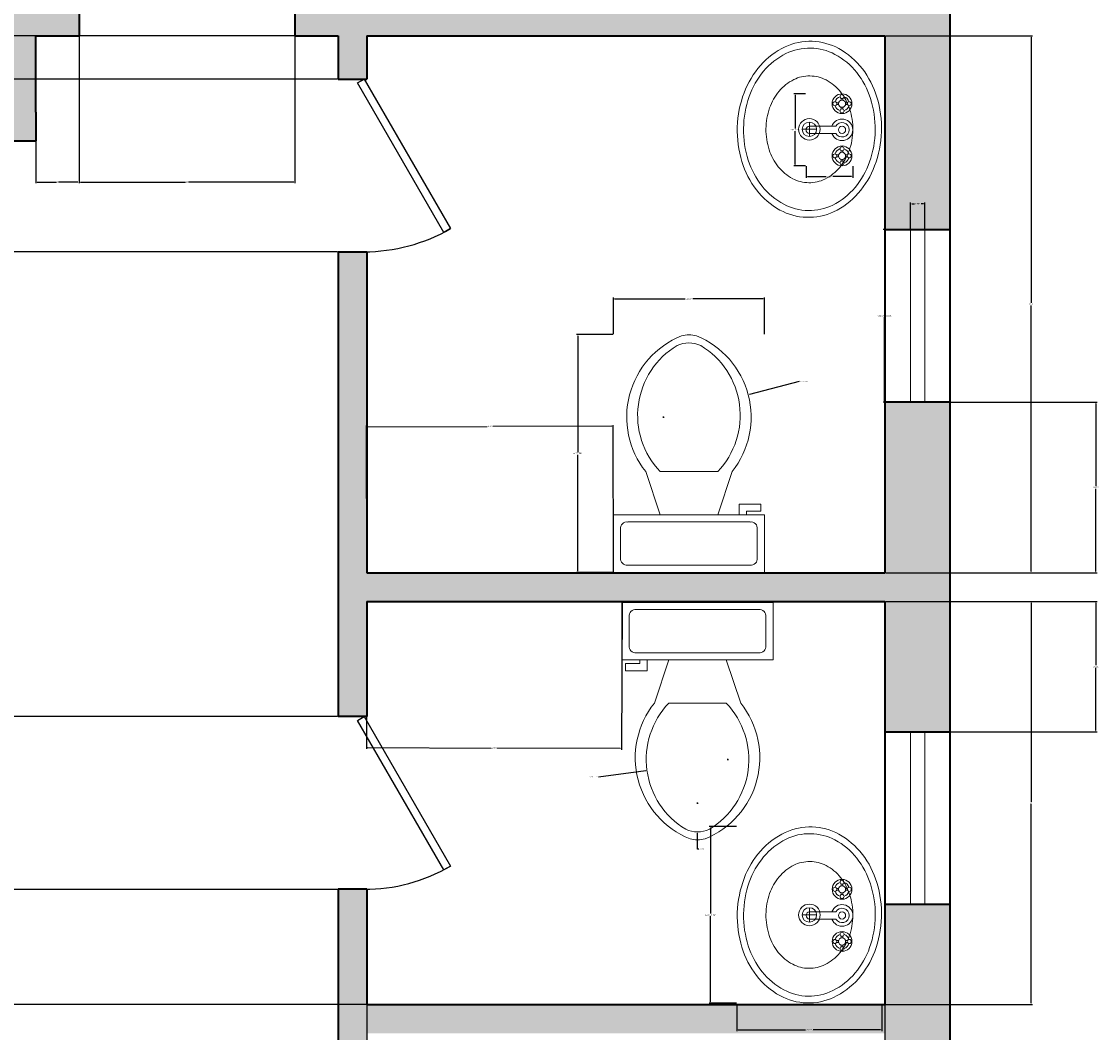
# Model space of a CAD drawing. Units: inches. Extents: x 1984 to 2284, y 2002 to 2421.
# Tile 3 of 4: x 2134 to 2284, y 2144 to 2285. Entities that reach past the tile are written whole.
import ezdxf

# ---------------------------------------------------------------- set-up
doc = ezdxf.new("R2010")
doc.units = ezdxf.units.IN
for name, color, linetype, lineweight in [('A-ANNO-DIMS', 2, 'Continuous', 18), ('A-DOOR', 3, 'Continuous', 25), ('A-FLOR-FIXT', 8, 'Continuous', 18), ('A-GLAZ', 4, 'Continuous', 18), ('A-WALL', 7, 'Continuous', 35)]:
    doc.layers.add(name, color=color, linetype=linetype, lineweight=lineweight)
doc.layers.add('A-WALL-PATT', color=18, linetype='Continuous', lineweight=13, true_color=0x000000)
doc.styles.get("Standard").update_dxf_attribs({"font": 'arial.ttf'})
doc.dimstyles.get("Standard").update_dxf_attribs({"dimtxt": 0.18, "dimasz": 0.18, "dimexe": 0.18, "dimexo": 0.0625, "dimgap": 0.09, "dimtad": 0, "dimtih": 1, "dimtoh": 1, "dimdec": 4, "dimzin": 0, "dimdsep": 46, "dimtxsty": 'Standard', "dimcen": 0.09, "dimadec": 0, "dimazin": 0, "dimtfac": 1, "dimtdec": 4, "dimtofl": 0, "dimtmove": 0, "dimatfit": 3, "dimfxl": 1, "dimtolj": 1, "dimtzin": 0, "dimarcsym": 0})

# ---------------------------------------------------------------- blocks, each defined once
blk = doc.blocks.new('Toilet - top')
for p, q in [((9.5, -6), (9.5, -2)), ((-10, -8.5), (-8, -8.5)), ((-10, -9.5), (-10, -8.5)), ((-8, -8.5), (-8, -8)), ((-7, -8), (-7, -9.5)), ((-4, -8), (-6, -14)), ((4, -8), (6, -14)), ((-7, -9.5), (-10, -9.5)), ((4, -14), (-4, -14))]:
    blk.add_line(p, q)
blk.add_lwpolyline([(10.5, -8), (10.5, 0), (-10.5, 0), (-10.5, -8)], close=True)
for points in [[(8.5, -1), (-8.5, -1)], [(-9.5, -2), (-9.5, -6)], [(-8.5, -7), (8.5, -7)]]:
    blk.add_lwpolyline(points)
for centre, radius, start, end in [((-8.62, -1.88), 0.884, 81.8699, 188.1301), ((8.62, -1.88), 0.884, 351.8699, 98.1301), ((-8.62, -6.12), 0.884, 171.8699, 278.1301), ((8.62, -6.12), 0.884, 261.8699, 8.1301), ((3.52, -21.58), 12.17, 141.4691, 247.9714), ((4.2, -21.82), 11.33, 136.3677, 238.9468), ((-3.52, -21.58), 12.17, 292.0284, 38.5307), ((-4.2, -21.82), 11.33, 301.053, 43.6321), ((0, -27.88), 4, 245.7318, 294.2682), ((0, -29), 4, 254.8605, 285.1395)]:
    blk.add_arc(centre, radius, start, end)
blk = doc.blocks.new('Sink - Oval top')
for p, q in [((-1, 0), (1, 0)), ((0, 1), (0, -1))]:
    blk.add_line(p, q)
for points in [[(-12.23, 0.39, 0.117634), (-11.46, -3.36, 0.104469), (-8.88, -6.8, 0.090016), (-5.08, -9.07, 0.08192), (-0.32, -10.02, 0.08192), (4.49, -9.38, 0.090016), (8.42, -7.36, 0.104469), (11.22, -4.09, 0.117634), (12.23, -0.39, 0.117634), (11.46, 3.36, 0.104469), (8.88, 6.8, 0.090016), (5.08, 9.07, 0.08192), (0.32, 10.02, 0.08192), (-4.49, 9.38, 0.090016), (-8.42, 7.36, 0.104469), (-11.22, 4.09, 0.117634)], [(-11.29, 0.16, 0.118622), (-10.52, -3.25, 0.104678), (-8.07, -6.36, 0.089562), (-4.54, -8.37, 0.081185), (-0.13, -9.15, 0.081185), (4.3, -8.49, 0.089562), (7.89, -6.58, 0.104678), (10.42, -3.55, 0.118622), (11.29, -0.16, 0.118622), (10.52, 3.25, 0.104678), (8.07, 6.36, 0.089562), (4.54, 8.37, 0.081185), (0.13, 9.15, 0.081185), (-4.3, 8.49, 0.089562), (-7.89, 6.58, 0.104678), (-10.42, 3.55, 0.118622)], [(-7.42, 0.08, 0.118283), (-6.91, -2.17, 0.104607), (-5.29, -4.21, 0.089718), (-2.97, -5.53, 0.081436), (-0.07, -6.04, 0.081436), (2.84, -5.59, 0.089718), (5.2, -4.33, 0.104607), (6.86, -2.32, 0.118283), (7.42, -0.08, 0.118283), (6.91, 2.17, 0.104607), (5.29, 4.21, 0.089718), (2.97, 5.53, 0.081436), (0.07, 6.04, 0.081436), (-2.84, 5.59, 0.089718), (-5.2, 4.33, 0.104607), (-6.86, 2.32, 0.118283)]]:
    blk.add_lwpolyline(points, format="xyb", close=True)
for radius in [1.5, 1]:
    blk.add_circle((0, 0), radius)
blk = doc.blocks.new('Faucet - Bathroom top')
for p, q in [((-4.107, 0.125), (-4.375, 0.125)), ((-3.75, 0.4788), (-3.75, 0.75)), ((-3.5, 0.482), (-3.5, 0.75)), ((-3.1461, 0.125), (-2.875, 0.125)), ((3.143, 0.125), (2.875, 0.125)), ((3.5, 0.4788), (3.5, 0.75)), ((3.75, 0.482), (3.75, 0.75)), ((4.1039, 0.125), (4.375, 0.125)), ((-4.1039, -0.125), (-4.375, -0.125)), ((-3.75, -0.4821), (-3.75, -0.75)), ((-3.5, -0.4789), (-3.5, -0.75)), ((-3.143, -0.125), (-2.875, -0.125)), ((-0.5, -0.8639), (-0.5, -4.5)), ((0.5, -4.5), (0.5, -0.8631)), ((3.1461, -0.125), (2.875, -0.125)), ((3.5, -0.4821), (3.5, -0.75)), ((3.75, -0.4789), (3.75, -0.75)), ((4.107, -0.125), (4.375, -0.125))]:
    blk.add_line(p, q)
for centre, radius in [((-3.625, 0), 1.375), ((-4.625, 0), 0.2795), ((-3.625, 0), 0.5), ((-3.625, 1), 0.2795), ((-2.625, 0), 0.2795), ((0, 0), 0.5), ((3.625, 0), 1.375), ((2.625, 0), 0.2795), ((3.625, 0), 0.5), ((3.625, 1), 0.2795), ((4.625, 0), 0.2795), ((-3.625, -1), 0.2795), ((3.625, -1), 0.2795)]:
    blk.add_circle(centre, radius)
for centre, radius, start, end in [((0, 0), 1.5, 289.6514, 250.3603), ((-3.625, 0), 1, 105.2407, 164.2093), ((-3.625, 0), 1, 16.44125, 74.07887), ((0, 0), 1, 300.3431, 239.7554), ((3.625, 0), 1, 106.12, 164.0884), ((3.625, 0), 1, 16.23422, 73.90469), ((-3.625, 0), 1, 196.2342, 253.9047), ((-3.625, 0), 1, 286.12, 344.0884), ((3.625, 0), 1, 196.4413, 254.0789), ((3.625, 0), 1, 285.2407, 344.2093), ((0, -4.5), 0.5, 180, 0)]:
    blk.add_arc(centre, radius, start, end)
blk = doc.blocks.new('*U10')
for p, q in [((0, 0), (0, -6)), ((40, 0), (40, -6))]:
    blk.add_line(p, q)
blk.add_lwpolyline([(0, 0), (34.64, 20), (35.52, 18.48), (0.87, -1.52)], close=True)
blk.add_arc((0, 0), 40, 0, 30)
blk = doc.blocks.new('GLAZING-24IN')
for p, q in [((0, 0), (0, 24)), ((2, 0), (2, 24))]:
    blk.add_line(p, q)
blk = doc.blocks.new('*D19')
at = {"layer": 'A-ANNO-DIMS', "color": 0, "lineweight": -2, "transparency": 16777216}
for p, q in [((2257.38, 2255.6), (2253.66, 2255.6)), ((2253.84, 2255.42), (2253.84, 2243.78)), ((2253.84, 2231.78), (2253.84, 2243.42)), ((2257.38, 2231.6), (2253.66, 2231.6))]:
    blk.add_line(p, q, dxfattribs=at)
at = {"layer": 'A-ANNO-DIMS', "color": 0, "transparency": 16777216}
for points in [[(2253.81, 2255.42), (2253.87, 2255.42), (2253.84, 2255.6)], [(2253.81, 2231.78), (2253.87, 2231.78), (2253.84, 2231.6)]]:
    blk.add_solid(points, dxfattribs=at)
at = {"layer": 'Defpoints', "color": 0, "transparency": 16777216}
for p in [(2253.84, 2255.6), (2257.44, 2255.6), (2257.44, 2231.6)]:
    blk.add_point(p, dxfattribs=at)
at = {"layer": 'A-ANNO-DIMS', "color": 0, "transparency": 16777216, "insert": (2253.84, 2243.6), "char_height": 0.18, "attachment_point": 5}
blk.add_mtext('\\A1;WINDOW 24 TYP.', dxfattribs=at)
blk = doc.blocks.new('*D20')
at = {"layer": 'A-ANNO-DIMS', "color": 0, "lineweight": -2, "transparency": 16777216}
for p, q in [((2257.44, 2255.66), (2257.44, 2259.38)), ((2257.62, 2259.2), (2257.98, 2259.2)), ((2259.26, 2259.2), (2258.9, 2259.2)), ((2259.44, 2255.66), (2259.44, 2259.38))]:
    blk.add_line(p, q, dxfattribs=at)
at = {"layer": 'A-ANNO-DIMS', "color": 0, "transparency": 16777216}
for points in [[(2257.62, 2259.23), (2257.62, 2259.17), (2257.44, 2259.2)], [(2259.26, 2259.23), (2259.26, 2259.17), (2259.44, 2259.2)]]:
    blk.add_solid(points, dxfattribs=at)
at = {"layer": 'Defpoints', "color": 0, "transparency": 16777216}
for p in [(2259.44, 2259.2), (2257.44, 2255.6), (2259.44, 2255.6)]:
    blk.add_point(p, dxfattribs=at)
at = {"layer": 'A-ANNO-DIMS', "color": 0, "transparency": 16777216, "insert": (2258.44, 2259.2), "char_height": 0.18, "attachment_point": 5}
blk.add_mtext('\\A1;2 TYP.', dxfattribs=at)
blk = doc.blocks.new('*D29')
at = {"layer": 'A-ANNO-DIMS', "color": 0, "lineweight": -2, "transparency": 16777216}
for p, q in [((2216.08, 2241.01), (2211, 2241.01)), ((2211.18, 2240.83), (2211.18, 2224.67)), ((2211.18, 2208.14), (2211.18, 2224.3)), ((2216.08, 2207.96), (2211, 2207.96))]:
    blk.add_line(p, q, dxfattribs=at)
at = {"layer": 'A-ANNO-DIMS', "color": 0, "transparency": 16777216}
for points in [[(2211.15, 2240.83), (2211.21, 2240.83), (2211.18, 2241.01)], [(2211.15, 2208.14), (2211.21, 2208.14), (2211.18, 2207.96)]]:
    blk.add_solid(points, dxfattribs=at)
at = {"layer": 'Defpoints', "color": 0, "transparency": 16777216}
for p in [(2216.14, 2241.01), (2211.18, 2207.96), (2216.14, 2207.96)]:
    blk.add_point(p, dxfattribs=at)
at = {"layer": 'A-ANNO-DIMS', "color": 0, "transparency": 16777216, "insert": (2211.18, 2224.49), "char_height": 0.18, "attachment_point": 5}
blk.add_mtext('\\A1;WC 33 TYP.', dxfattribs=at)
blk = doc.blocks.new('*D30')
at = {"layer": 'A-ANNO-DIMS', "color": 0, "lineweight": -2, "transparency": 16777216}
for p, q in [((2216.14, 2241.07), (2216.14, 2246.15)), ((2216.32, 2245.97), (2226.11, 2245.97)), ((2236.96, 2245.97), (2227.17, 2245.97)), ((2237.14, 2241.07), (2237.14, 2246.15))]:
    blk.add_line(p, q, dxfattribs=at)
at = {"layer": 'A-ANNO-DIMS', "color": 0, "transparency": 16777216}
for points in [[(2216.32, 2246), (2216.32, 2245.94), (2216.14, 2245.97)], [(2236.96, 2246), (2236.96, 2245.94), (2237.14, 2245.97)]]:
    blk.add_solid(points, dxfattribs=at)
at = {"layer": 'Defpoints', "color": 0, "transparency": 16777216}
for p in [(2216.14, 2245.97), (2216.14, 2241.01), (2237.14, 2241.01)]:
    blk.add_point(p, dxfattribs=at)
at = {"layer": 'A-ANNO-DIMS', "color": 0, "transparency": 16777216, "insert": (2226.64, 2245.97), "char_height": 0.18, "attachment_point": 5}
blk.add_mtext('\\A1;21 TYP.', dxfattribs=at)
blk = doc.blocks.new('*D31')
at = {"layer": 'A-ANNO-DIMS', "color": 0, "lineweight": -2, "transparency": 16777216}
for p, q in [((2233.26, 2172.63), (2229.46, 2172.63)), ((2229.64, 2172.45), (2229.64, 2160.54)), ((2229.64, 2148.26), (2229.64, 2160.17)), ((2233.26, 2148.08), (2229.46, 2148.08))]:
    blk.add_line(p, q, dxfattribs=at)
at = {"layer": 'A-ANNO-DIMS', "color": 0, "transparency": 16777216}
for points in [[(2229.61, 2172.45), (2229.67, 2172.45), (2229.64, 2172.63)], [(2229.61, 2148.26), (2229.67, 2148.26), (2229.64, 2148.08)]]:
    blk.add_solid(points, dxfattribs=at)
at = {"layer": 'Defpoints', "color": 0, "transparency": 16777216}
for p in [(2233.32, 2172.63), (2229.64, 2148.08), (2233.32, 2148.08)]:
    blk.add_point(p, dxfattribs=at)
at = {"layer": 'A-ANNO-DIMS', "color": 0, "transparency": 16777216, "insert": (2229.64, 2160.36), "char_height": 0.18, "attachment_point": 5}
blk.add_mtext('\\A1;BASIN 25 TYP.', dxfattribs=at)
blk = doc.blocks.new('*D32')
at = {"layer": 'A-ANNO-DIMS', "color": 0, "lineweight": -2, "transparency": 16777216}
for p, q in [((2233.32, 2148.02), (2233.32, 2144.22)), ((2253.46, 2148.02), (2253.46, 2144.22)), ((2233.5, 2144.4), (2242.86, 2144.4)), ((2253.28, 2144.4), (2243.92, 2144.4))]:
    blk.add_line(p, q, dxfattribs=at)
at = {"layer": 'A-ANNO-DIMS', "color": 0, "transparency": 16777216}
for points in [[(2233.5, 2144.43), (2233.5, 2144.37), (2233.32, 2144.4)], [(2253.28, 2144.43), (2253.28, 2144.37), (2253.46, 2144.4)]]:
    blk.add_solid(points, dxfattribs=at)
at = {"layer": 'Defpoints', "color": 0, "transparency": 16777216}
for p in [(2233.32, 2148.08), (2253.46, 2148.08), (2253.46, 2144.4)]:
    blk.add_point(p, dxfattribs=at)
at = {"layer": 'A-ANNO-DIMS', "color": 0, "transparency": 16777216, "insert": (2243.39, 2144.4), "char_height": 0.18, "attachment_point": 5}
blk.add_mtext('\\A1;20 TYP.', dxfattribs=at)
blk = doc.blocks.new('*D33')
at = {"layer": 'A-ANNO-DIMS', "color": 0, "lineweight": -2, "transparency": 16777216}
for p, q in [((2242.86, 2274.47), (2241.24, 2274.47)), ((2241.42, 2274.29), (2241.42, 2269.65)), ((2241.42, 2264.65), (2241.42, 2269.29)), ((2242.86, 2264.47), (2241.24, 2264.47))]:
    blk.add_line(p, q, dxfattribs=at)
at = {"layer": 'A-ANNO-DIMS', "color": 0, "transparency": 16777216}
for points in [[(2241.39, 2274.29), (2241.45, 2274.29), (2241.42, 2274.47)], [(2241.39, 2264.65), (2241.45, 2264.65), (2241.42, 2264.47)]]:
    blk.add_solid(points, dxfattribs=at)
at = {"layer": 'Defpoints', "color": 0, "transparency": 16777216}
for p in [(2242.92, 2274.47), (2241.42, 2264.47), (2242.92, 2264.47)]:
    blk.add_point(p, dxfattribs=at)
at = {"layer": 'A-ANNO-DIMS', "color": 0, "transparency": 16777216, "insert": (2241.42, 2269.47), "char_height": 0.18, "attachment_point": 5}
blk.add_mtext('\\A1;TAP 10 TYP.', dxfattribs=at)
blk = doc.blocks.new('*D34')
at = {"layer": 'A-ANNO-DIMS', "color": 0, "lineweight": -2, "transparency": 16777216}
for p, q in [((2242.92, 2264.41), (2242.92, 2262.79)), ((2249.42, 2264.41), (2249.42, 2262.79)), ((2243.1, 2262.97), (2245.71, 2262.97)), ((2249.24, 2262.97), (2246.63, 2262.97))]:
    blk.add_line(p, q, dxfattribs=at)
at = {"layer": 'A-ANNO-DIMS', "color": 0, "transparency": 16777216}
for points in [[(2243.1, 2263), (2243.1, 2262.94), (2242.92, 2262.97)], [(2249.24, 2263), (2249.24, 2262.94), (2249.42, 2262.97)]]:
    blk.add_solid(points, dxfattribs=at)
at = {"layer": 'Defpoints', "color": 0, "transparency": 16777216}
for p in [(2242.92, 2264.47), (2249.42, 2264.47), (2249.42, 2262.97)]:
    blk.add_point(p, dxfattribs=at)
at = {"layer": 'A-ANNO-DIMS', "color": 0, "transparency": 16777216, "insert": (2246.17, 2262.97), "char_height": 0.18, "attachment_point": 5}
blk.add_mtext('\\A1;7 TYP.', dxfattribs=at)
blk = doc.blocks.new('*D51')
at = {"layer": 'A-ANNO-DIMS', "color": 0, "lineweight": -2, "transparency": 16777216}
for p, q in [((2253.95, 2282.51), (2274.37, 2282.51)), ((2274.19, 2282.33), (2274.19, 2245.4)), ((2274.19, 2208.09), (2274.19, 2245.03)), ((2253.95, 2207.91), (2274.37, 2207.91))]:
    blk.add_line(p, q, dxfattribs=at)
at = {"layer": 'A-ANNO-DIMS', "color": 0, "transparency": 16777216}
for points in [[(2274.16, 2282.33), (2274.22, 2282.33), (2274.19, 2282.51)], [(2274.16, 2208.09), (2274.22, 2208.09), (2274.19, 2207.91)]]:
    blk.add_solid(points, dxfattribs=at)
at = {"layer": 'Defpoints', "color": 0, "transparency": 16777216}
for p in [(2253.89, 2282.51), (2253.89, 2207.91), (2274.19, 2207.91)]:
    blk.add_point(p, dxfattribs=at)
at = {"layer": 'A-ANNO-DIMS', "color": 0, "transparency": 16777216, "insert": (2274.19, 2245.21), "char_height": 0.18, "attachment_point": 5}
blk.add_mtext('\\A1;74.6', dxfattribs=at)
blk = doc.blocks.new('*D52')
at = {"layer": 'A-ANNO-DIMS', "color": 0, "lineweight": -2, "transparency": 16777216}
for p, q in [((2253.95, 2203.91), (2274.37, 2203.91)), ((2274.19, 2203.73), (2274.19, 2176.09)), ((2274.19, 2148.09), (2274.19, 2175.73)), ((2253.95, 2147.91), (2274.37, 2147.91))]:
    blk.add_line(p, q, dxfattribs=at)
at = {"layer": 'A-ANNO-DIMS', "color": 0, "transparency": 16777216}
for points in [[(2274.16, 2203.73), (2274.22, 2203.73), (2274.19, 2203.91)], [(2274.16, 2148.09), (2274.22, 2148.09), (2274.19, 2147.91)]]:
    blk.add_solid(points, dxfattribs=at)
at = {"layer": 'Defpoints', "color": 0, "transparency": 16777216}
for p in [(2253.89, 2203.91), (2253.89, 2147.91), (2274.19, 2147.91)]:
    blk.add_point(p, dxfattribs=at)
at = {"layer": 'A-ANNO-DIMS', "color": 0, "transparency": 16777216, "insert": (2274.19, 2175.91), "char_height": 0.18, "attachment_point": 5}
blk.add_mtext('\\A1;56', dxfattribs=at)
blk = doc.blocks.new('*D54')
at = {"layer": 'A-ANNO-DIMS', "color": 0, "lineweight": -2, "transparency": 16777216}
for p, q in [((2181.89, 2147.85), (2181.89, 2127.43)), ((2253.89, 2147.85), (2253.89, 2127.43)), ((2182.07, 2127.61), (2217.67, 2127.61)), ((2253.71, 2127.61), (2218.1, 2127.61))]:
    blk.add_line(p, q, dxfattribs=at)
at = {"layer": 'A-ANNO-DIMS', "color": 0, "transparency": 16777216}
for points in [[(2182.07, 2127.64), (2182.07, 2127.58), (2181.89, 2127.61)], [(2253.71, 2127.64), (2253.71, 2127.58), (2253.89, 2127.61)]]:
    blk.add_solid(points, dxfattribs=at)
at = {"layer": 'Defpoints', "color": 0, "transparency": 16777216}
for p in [(2181.89, 2147.91), (2253.89, 2147.91), (2181.89, 2127.61)]:
    blk.add_point(p, dxfattribs=at)
at = {"layer": 'A-ANNO-DIMS', "color": 0, "transparency": 16777216, "insert": (2217.89, 2127.61), "char_height": 0.18, "attachment_point": 5}
blk.add_mtext('\\A1;72', dxfattribs=at)
blk = doc.blocks.new('*D61')
at = {"layer": 'A-ANNO-DIMS', "color": 0, "lineweight": -2, "transparency": 16777216}
for p, q in [((2253.95, 2231.6), (2283.37, 2231.6)), ((2283.19, 2231.42), (2283.19, 2219.94)), ((2283.19, 2208.09), (2283.19, 2219.57)), ((2253.95, 2207.91), (2283.37, 2207.91))]:
    blk.add_line(p, q, dxfattribs=at)
at = {"layer": 'A-ANNO-DIMS', "color": 0, "transparency": 16777216}
for points in [[(2283.16, 2231.42), (2283.22, 2231.42), (2283.19, 2231.6)], [(2283.16, 2208.09), (2283.22, 2208.09), (2283.19, 2207.91)]]:
    blk.add_solid(points, dxfattribs=at)
at = {"layer": 'Defpoints', "color": 0, "transparency": 16777216}
for p in [(2253.89, 2231.6), (2253.89, 2207.91), (2283.19, 2207.91)]:
    blk.add_point(p, dxfattribs=at)
at = {"layer": 'A-ANNO-DIMS', "color": 0, "transparency": 16777216, "insert": (2283.19, 2219.76), "char_height": 0.18, "attachment_point": 5}
blk.add_mtext('\\A1;23.687', dxfattribs=at)
blk = doc.blocks.new('*D62')
at = {"layer": 'A-ANNO-DIMS', "color": 0, "lineweight": -2, "transparency": 16777216}
for p, q in [((2253.95, 2203.91), (2283.37, 2203.91)), ((2283.19, 2203.73), (2283.19, 2195.05)), ((2283.19, 2185.99), (2283.19, 2194.68)), ((2253.95, 2185.81), (2283.37, 2185.81))]:
    blk.add_line(p, q, dxfattribs=at)
at = {"layer": 'A-ANNO-DIMS', "color": 0, "transparency": 16777216}
for points in [[(2283.16, 2203.73), (2283.22, 2203.73), (2283.19, 2203.91)], [(2283.16, 2185.99), (2283.22, 2185.99), (2283.19, 2185.81)]]:
    blk.add_solid(points, dxfattribs=at)
at = {"layer": 'Defpoints', "color": 0, "transparency": 16777216}
for p in [(2253.89, 2203.91), (2253.89, 2185.81), (2283.19, 2185.81)]:
    blk.add_point(p, dxfattribs=at)
at = {"layer": 'A-ANNO-DIMS', "color": 0, "transparency": 16777216, "insert": (2283.19, 2194.86), "char_height": 0.18, "attachment_point": 5}
blk.add_mtext('\\A1;18.098', dxfattribs=at)
blk = doc.blocks.new('*D65')
at = {"layer": 'A-ANNO-DIMS', "color": 0, "lineweight": -2, "transparency": 16777216}
for p, q in [((2135.89, 2282.45), (2135.89, 2262.03)), ((2141.89, 2282.45), (2141.89, 2262.03)), ((2136.07, 2262.21), (2138.74, 2262.21)), ((2141.71, 2262.21), (2139.03, 2262.21))]:
    blk.add_line(p, q, dxfattribs=at)
at = {"layer": 'A-ANNO-DIMS', "color": 0, "transparency": 16777216}
for points in [[(2136.07, 2262.24), (2136.07, 2262.18), (2135.89, 2262.21)], [(2141.71, 2262.24), (2141.71, 2262.18), (2141.89, 2262.21)]]:
    blk.add_solid(points, dxfattribs=at)
at = {"layer": 'Defpoints', "color": 0, "transparency": 16777216}
for p in [(2135.89, 2282.51), (2141.89, 2282.51), (2135.89, 2262.21)]:
    blk.add_point(p, dxfattribs=at)
at = {"layer": 'A-ANNO-DIMS', "color": 0, "transparency": 16777216, "insert": (2138.89, 2262.21), "char_height": 0.18, "attachment_point": 5}
blk.add_mtext('\\A1;6', dxfattribs=at)
blk = doc.blocks.new('*D66')
at = {"layer": 'A-ANNO-DIMS', "color": 0, "lineweight": -2, "transparency": 16777216}
for p, q in [((2141.89, 2282.45), (2141.89, 2262.03)), ((2171.89, 2282.45), (2171.89, 2262.03)), ((2142.07, 2262.21), (2156.67, 2262.21)), ((2171.71, 2262.21), (2157.1, 2262.21))]:
    blk.add_line(p, q, dxfattribs=at)
at = {"layer": 'A-ANNO-DIMS', "color": 0, "transparency": 16777216}
for points in [[(2142.07, 2262.24), (2142.07, 2262.18), (2141.89, 2262.21)], [(2171.71, 2262.24), (2171.71, 2262.18), (2171.89, 2262.21)]]:
    blk.add_solid(points, dxfattribs=at)
at = {"layer": 'Defpoints', "color": 0, "transparency": 16777216}
for p in [(2141.89, 2282.51), (2171.89, 2282.51), (2141.89, 2262.21)]:
    blk.add_point(p, dxfattribs=at)
at = {"layer": 'A-ANNO-DIMS', "color": 0, "transparency": 16777216, "insert": (2156.89, 2262.21), "char_height": 0.18, "attachment_point": 5}
blk.add_mtext('\\A1;30', dxfattribs=at)
blk = doc.blocks.new('*D69')
at = {"layer": 'A-ANNO-DIMS', "color": 0, "lineweight": -2, "transparency": 16777216}
for p, q in [((2177.82, 2276.51), (1984.41, 2276.51)), ((1984.59, 2276.33), (1984.59, 2264.69)), ((1984.59, 2252.69), (1984.59, 2264.33)), ((2177.82, 2252.51), (1984.41, 2252.51))]:
    blk.add_line(p, q, dxfattribs=at)
at = {"layer": 'A-ANNO-DIMS', "color": 0, "transparency": 16777216}
for points in [[(1984.56, 2276.33), (1984.62, 2276.33), (1984.59, 2276.51)], [(1984.56, 2252.69), (1984.62, 2252.69), (1984.59, 2252.51)]]:
    blk.add_solid(points, dxfattribs=at)
at = {"layer": 'Defpoints', "color": 0, "transparency": 16777216}
for p in [(1984.59, 2276.51), (2177.89, 2276.51), (2177.89, 2252.51)]:
    blk.add_point(p, dxfattribs=at)
at = {"layer": 'A-ANNO-DIMS', "color": 0, "transparency": 16777216, "insert": (1984.59, 2264.51), "char_height": 0.18, "attachment_point": 5}
blk.add_mtext('\\A1;24', dxfattribs=at)
blk = doc.blocks.new('*D70')
at = {"layer": 'A-ANNO-DIMS', "color": 0, "lineweight": -2, "transparency": 16777216}
for p, q in [((2177.82, 2282.51), (1984.41, 2282.51)), ((1984.59, 2282.33), (1984.59, 2279.7)), ((1984.59, 2276.69), (1984.59, 2279.33)), ((2177.82, 2276.51), (1984.41, 2276.51))]:
    blk.add_line(p, q, dxfattribs=at)
at = {"layer": 'A-ANNO-DIMS', "color": 0, "transparency": 16777216}
for points in [[(1984.56, 2282.33), (1984.62, 2282.33), (1984.59, 2282.51)], [(1984.56, 2276.69), (1984.62, 2276.69), (1984.59, 2276.51)]]:
    blk.add_solid(points, dxfattribs=at)
at = {"layer": 'Defpoints', "color": 0, "transparency": 16777216}
for p in [(1984.59, 2282.51), (2177.89, 2282.51), (2177.89, 2276.51)]:
    blk.add_point(p, dxfattribs=at)
at = {"layer": 'A-ANNO-DIMS', "color": 0, "transparency": 16777216, "insert": (1984.59, 2279.51), "char_height": 0.18, "attachment_point": 5}
blk.add_mtext('\\A1;6', dxfattribs=at)
blk = doc.blocks.new('*D71')
at = {"layer": 'A-ANNO-DIMS', "color": 0, "lineweight": -2, "transparency": 16777216}
for p, q in [((2177.82, 2187.91), (1984.41, 2187.91)), ((1984.59, 2187.73), (1984.59, 2176.09)), ((1984.59, 2164.09), (1984.59, 2175.73)), ((2177.82, 2163.91), (1984.41, 2163.91))]:
    blk.add_line(p, q, dxfattribs=at)
at = {"layer": 'A-ANNO-DIMS', "color": 0, "transparency": 16777216}
for points in [[(1984.56, 2187.73), (1984.62, 2187.73), (1984.59, 2187.91)], [(1984.56, 2164.09), (1984.62, 2164.09), (1984.59, 2163.91)]]:
    blk.add_solid(points, dxfattribs=at)
at = {"layer": 'Defpoints', "color": 0, "transparency": 16777216}
for p in [(1984.59, 2187.91), (2177.89, 2187.91), (2177.89, 2163.91)]:
    blk.add_point(p, dxfattribs=at)
at = {"layer": 'A-ANNO-DIMS', "color": 0, "transparency": 16777216, "insert": (1984.59, 2175.91), "char_height": 0.18, "attachment_point": 5}
blk.add_mtext('\\A1;24', dxfattribs=at)
blk = doc.blocks.new('*D72')
at = {"layer": 'A-ANNO-DIMS', "color": 0, "lineweight": -2, "transparency": 16777216}
for p, q in [((2181.82, 2163.91), (1984.41, 2163.91)), ((1984.59, 2163.73), (1984.59, 2156.09)), ((1984.59, 2148.09), (1984.59, 2155.73)), ((2181.82, 2147.91), (1984.41, 2147.91))]:
    blk.add_line(p, q, dxfattribs=at)
at = {"layer": 'A-ANNO-DIMS', "color": 0, "transparency": 16777216}
for points in [[(1984.56, 2163.73), (1984.62, 2163.73), (1984.59, 2163.91)], [(1984.56, 2148.09), (1984.62, 2148.09), (1984.59, 2147.91)]]:
    blk.add_solid(points, dxfattribs=at)
at = {"layer": 'Defpoints', "color": 0, "transparency": 16777216}
for p in [(1984.59, 2163.91), (2181.89, 2163.91), (2181.89, 2147.91)]:
    blk.add_point(p, dxfattribs=at)
at = {"layer": 'A-ANNO-DIMS', "color": 0, "transparency": 16777216, "insert": (1984.59, 2155.91), "char_height": 0.18, "attachment_point": 5}
blk.add_mtext('\\A1;16', dxfattribs=at)
blk = doc.blocks.new('*D80')
at = {"layer": 'A-ANNO-DIMS', "color": 0, "lineweight": -2, "transparency": 16777216}
for p, q in [((2181.89, 2207.97), (2181.85, 2228.39)), ((2182.03, 2228.21), (2198.59, 2228.24)), ((2215.93, 2228.26), (2199.38, 2228.24)), ((2216.14, 2208.03), (2216.11, 2228.44))]:
    blk.add_line(p, q, dxfattribs=at)
at = {"layer": 'A-ANNO-DIMS', "color": 0, "transparency": 16777216}
for points in [[(2182.03, 2228.24), (2182.03, 2228.18), (2181.85, 2228.21)], [(2215.93, 2228.29), (2215.93, 2228.23), (2216.11, 2228.26)]]:
    blk.add_solid(points, dxfattribs=at)
at = {"layer": 'Defpoints', "color": 0, "transparency": 16777216}
for p in [(2216.11, 2228.26), (2181.89, 2207.91), (2216.14, 2207.96)]:
    blk.add_point(p, dxfattribs=at)
at = {"layer": 'A-ANNO-DIMS', "color": 0, "transparency": 16777216, "insert": (2198.98, 2228.24), "char_height": 0.18, "attachment_point": 5}
blk.add_mtext('\\A1;34.26', dxfattribs=at)
blk = doc.blocks.new('*D81')
at = {"layer": 'A-ANNO-DIMS', "color": 0, "lineweight": -2, "transparency": 16777216}
for p, q in [((2181.89, 2203.85), (2181.81, 2183.43)), ((2217.34, 2203.72), (2217.26, 2183.3)), ((2181.99, 2183.61), (2199.14, 2183.55)), ((2217.08, 2183.48), (2199.93, 2183.55))]:
    blk.add_line(p, q, dxfattribs=at)
at = {"layer": 'A-ANNO-DIMS', "color": 0, "transparency": 16777216}
for points in [[(2181.99, 2183.64), (2181.99, 2183.58), (2181.81, 2183.61)], [(2217.08, 2183.51), (2217.08, 2183.45), (2217.26, 2183.48)]]:
    blk.add_solid(points, dxfattribs=at)
at = {"layer": 'Defpoints', "color": 0, "transparency": 16777216}
for p in [(2181.89, 2203.91), (2217.34, 2203.78), (2181.81, 2183.61)]:
    blk.add_point(p, dxfattribs=at)
at = {"layer": 'A-ANNO-DIMS', "color": 0, "transparency": 16777216, "insert": (2199.54, 2183.55), "char_height": 0.18, "attachment_point": 5}
blk.add_mtext('\\A1;35.45', dxfattribs=at)
blk = doc.blocks.new('*D83')
at = {"layer": 'A-ANNO-DIMS', "color": 0, "lineweight": -2, "transparency": 16777216}
for p, q in [((2241.95, 2234.49), (2235.07, 2232.68)), ((2223.03, 2229.54), (2223.21, 2229.54)), ((2223.12, 2229.45), (2223.12, 2229.63))]:
    blk.add_line(p, q, dxfattribs=at)
at = {"layer": 'A-ANNO-DIMS', "color": 0, "transparency": 16777216}
blk.add_solid([(2235.06, 2232.71), (2235.07, 2232.65), (2234.89, 2232.64)], dxfattribs=at)
at = {"layer": 'Defpoints', "color": 0, "transparency": 16777216}
for p in [(2234.89, 2232.64), (2223.12, 2229.54)]:
    blk.add_point(p, dxfattribs=at)
at = {"layer": 'A-ANNO-DIMS', "color": 0, "transparency": 16777216, "insert": (2242.63, 2234.49), "char_height": 0.18, "attachment_point": 5}
blk.add_mtext('\\A1;4X R12.17', dxfattribs=at)
blk = doc.blocks.new('*D84')
at = {"layer": 'A-ANNO-DIMS', "color": 0, "lineweight": -2, "transparency": 16777216}
for p, q in [((2231.95, 2181.97), (2232.13, 2181.97)), ((2232.04, 2181.88), (2232.04, 2182.06)), ((2214.07, 2179.55), (2220.63, 2180.43))]:
    blk.add_line(p, q, dxfattribs=at)
at = {"layer": 'A-ANNO-DIMS', "color": 0, "transparency": 16777216}
blk.add_solid([(2220.62, 2180.46), (2220.63, 2180.4), (2220.81, 2180.46)], dxfattribs=at)
at = {"layer": 'Defpoints', "color": 0, "transparency": 16777216}
for p in [(2232.04, 2181.97), (2220.81, 2180.46)]:
    blk.add_point(p, dxfattribs=at)
at = {"layer": 'A-ANNO-DIMS', "color": 0, "transparency": 16777216, "insert": (2213.39, 2179.55), "char_height": 0.18, "attachment_point": 5}
blk.add_mtext('\\A1;4X R11.33', dxfattribs=at)
blk = doc.blocks.new('*D85')
at = {"layer": 'A-ANNO-DIMS', "color": 0, "lineweight": -2, "transparency": 16777216}
for p, q in [((2227.75, 2175.91), (2227.93, 2175.91)), ((2227.84, 2175.82), (2227.84, 2176)), ((2227.84, 2169.51), (2227.84, 2171.73)), ((2228.02, 2169.51), (2227.84, 2169.51))]:
    blk.add_line(p, q, dxfattribs=at)
at = {"layer": 'A-ANNO-DIMS', "color": 0, "transparency": 16777216}
blk.add_solid([(2227.87, 2171.73), (2227.81, 2171.73), (2227.84, 2171.91)], dxfattribs=at)
at = {"layer": 'Defpoints', "color": 0, "transparency": 16777216}
for p in [(2227.84, 2175.91), (2227.84, 2171.91)]:
    blk.add_point(p, dxfattribs=at)
at = {"layer": 'A-ANNO-DIMS', "color": 0, "transparency": 16777216, "insert": (2228.45, 2169.51), "char_height": 0.18, "attachment_point": 5}
blk.add_mtext('\\A1;4X R4', dxfattribs=at)

msp = doc.modelspace()

# ---------------------------------------------------------------- hatches: boundary and pattern name
at = {"layer": 'A-WALL-PATT'}
h = msp.add_hatch(color=256, dxfattribs=at)
h.dxf.hatch_style = 1
h.paths.add_polyline_path([(2178.9401, 2400.9122), (2100.8198, 2400.9122), (2100.8198, 2391.9122), (2131.8852, 2391.9122), (2131.8852, 2271.9122), (2125.8852, 2271.9122), (2125.8852, 2267.9122), (2135.8852, 2267.9122), (2135.8852, 2271.9122), (2135.8852, 2282.5141), (2141.8852, 2282.5141), (2141.8852, 2286.5141), (2135.8852, 2286.5141), (2135.8852, 2391.9122), (2178.9401, 2391.9122)])
h = msp.add_hatch(color=256, dxfattribs=at)
h.dxf.hatch_style = 1
h.paths.add_polyline_path([(2262.8852, 2400.9122), (2226.9401, 2400.9122), (2226.9401, 2391.9122), (2253.8852, 2391.9122), (2253.8852, 2286.5141), (2171.8852, 2286.5141), (2171.8852, 2282.5141), (2177.8852, 2282.5141), (2177.8852, 2276.5141), (2181.8852, 2276.5141), (2181.8852, 2282.5141), (2253.8852, 2282.5141), (2253.8852, 2255.5995), (2262.8852, 2255.5995)])
h = msp.add_hatch(color=256, dxfattribs=at)
h.dxf.hatch_style = 1
h.paths.add_polyline_path([(2262.8852, 2231.5995), (2253.8852, 2231.5995), (2253.8852, 2207.9122), (2181.8852, 2207.9122), (2181.8852, 2252.5141), (2177.8852, 2252.5141), (2177.8852, 2207.9122), (2177.8852, 2187.9122), (2181.8852, 2187.9122), (2181.8852, 2203.9122), (2253.8852, 2203.9122), (2253.8852, 2185.8141), (2262.8852, 2185.8141)])
h = msp.add_hatch(color=256, dxfattribs=at)
h.dxf.hatch_style = 1
h.paths.add_polyline_path([(2262.8852, 2161.8141), (2253.8852, 2161.8141), (2253.8852, 2147.9122), (2181.8852, 2147.9122), (2181.8852, 2163.9122), (2177.8852, 2163.9122), (2177.8852, 2147.9122), (2177.8852, 2101.9122), (2171.8852, 2101.9122), (2171.8852, 2097.9122), (2177.8852, 2097.9122), (2181.8852, 2097.9122), (2181.8852, 2143.9122), (2253.8852, 2143.9122), (2253.8852, 2031.9122), (2225.8984, 2031.9122), (2225.8984, 2022.9122), (2262.8852, 2022.9122)])

# ---------------------------------------------------------------- linework, layer by layer
at = {"layer": 'A-WALL'}
for p, q in [((2141.8852, 2286.5141), (2141.8852, 2282.5141)), ((2171.8852, 2286.5141), (2171.8852, 2282.5141)), ((2135.8852, 2282.5141), (2141.8852, 2282.5141)), ((2135.8852, 2271.9122), (2135.8852, 2282.5141)), ((2171.8852, 2282.5141), (2177.8852, 2282.5141)), ((2177.8852, 2282.5141), (2177.8852, 2276.5141)), ((2181.8852, 2282.5141), (2181.8852, 2276.5141)), ((2181.8852, 2282.5141), (2253.8852, 2282.5141)), ((2253.8852, 2282.5141), (2253.8852, 2207.9122)), ((2177.8852, 2276.5141), (2181.8852, 2276.5141)), ((2135.8852, 2271.9122), (2135.8852, 2267.9122)), ((2125.8852, 2267.9122), (2135.8852, 2267.9122)), ((2177.8852, 2252.5141), (2181.8852, 2252.5141)), ((2177.8852, 2252.5141), (2177.8852, 2207.9122)), ((2181.8852, 2252.5141), (2181.8852, 2207.9122)), ((2177.8852, 2207.9122), (2177.8852, 2187.9122)), ((2181.8852, 2207.9122), (2253.8852, 2207.9122)), ((2181.8852, 2203.9122), (2253.8852, 2203.9122)), ((2181.8852, 2203.9122), (2181.8852, 2187.9122)), ((2253.8852, 2203.9122), (2253.8852, 2147.9122)), ((2181.8852, 2187.9122), (2177.8852, 2187.9122)), ((2181.8852, 2163.9122), (2177.8852, 2163.9122)), ((2177.8852, 2163.9122), (2177.8852, 2147.9122)), ((2181.8852, 2163.9122), (2181.8852, 2147.9122)), ((2177.8852, 2147.9122), (2177.8852, 2101.9122)), ((2181.8852, 2147.9122), (2253.8852, 2147.9122))]:
    msp.add_line(p, q, dxfattribs=at)
for points in [[(2019.8852, 2022.9122), (2004.8852, 2022.9122), (2004.8852, 2400.9122), (2262.8852, 2400.9122), (2262.8852, 2022.9122), (2055.8852, 2022.9122)], [(2253.8852, 2255.5995), (2262.8852, 2255.5995)], [(2262.8852, 2231.5995), (2253.8852, 2231.5995)], [(2253.8852, 2185.8141), (2262.8852, 2185.8141)], [(2262.8852, 2161.8141), (2253.8852, 2161.8141)]]:
    msp.add_lwpolyline(points, dxfattribs=at)

# ---------------------------------------------------------------- block references
at = {"layer": 'A-DOOR', "xscale": 0.75, "yscale": 0.75, "zscale": 0.75}
msp.add_blockref('*U10', (2141.8852, 2287.0141), dxfattribs=at)
at = {"layer": 'A-DOOR', "xscale": 0.6, "yscale": 0.6, "zscale": 0.6, "rotation": 270}
for p in [(2181.4852, 2276.5141), (2181.4852, 2187.9122)]:
    msp.add_blockref('*U10', p, dxfattribs=at)
at = {"layer": 'A-FLOR-FIXT'}
for name, p, rotation in [('Sink - Oval top', (2243.3822, 2269.5357), 270), ('Faucet - Bathroom top', (2247.919, 2269.468), 270), ('Toilet - top', (2226.6419, 2207.9636), 180), ('Sink - Oval top', (2243.3874, 2160.3561), 270), ('Faucet - Bathroom top', (2247.9242, 2160.2884), 270)]:
    msp.add_blockref(name, p, dxfattribs=dict(at, rotation=rotation))
msp.add_blockref('Toilet - top', (2227.8355, 2203.7838), dxfattribs=at)
at = {"layer": 'A-GLAZ'}
msp.add_blockref('GLAZING-24IN', (2257.4413, 2231.5995), dxfattribs=at)
at = {"layer": 'A-GLAZ', "rotation": 180}
msp.add_blockref('GLAZING-24IN', (2259.4413, 2185.8141), dxfattribs=at)

# ---------------------------------------------------------------- dimensions: what is measured, and where the dimension line sits
at = {"layer": 'A-ANNO-DIMS'}
for base, p1, p2, angle, override, picture, middle in [((1984.5852, 2282.5141), (2177.8852, 2276.5141), (2177.8852, 2282.5141), 90, {"dimdec": 0, "dimlfac": 1, "dimrnd": 0, "dimzin": 0, "dimdsep": 46, "dimlunit": 2}, '*D70', (1984.5852, 2279.5141)), ((2135.8852, 2262.2141), (2141.8852, 2282.5141), (2135.8852, 2282.5141), 180, {"dimdec": 0, "dimlfac": 1, "dimrnd": 0, "dimzin": 0, "dimdsep": 46, "dimlunit": 2}, '*D65', (2138.8852, 2262.2141)), ((2141.8852, 2262.2141), (2171.8852, 2282.5141), (2141.8852, 2282.5141), 180, {"dimdec": 0, "dimlfac": 1, "dimrnd": 0, "dimzin": 0, "dimdsep": 46, "dimlunit": 2}, '*D66', (2156.8852, 2262.2141)), ((2274.1852, 2207.9122), (2253.8852, 2282.5141), (2253.8852, 2207.9122), 270, {"dimdec": 1, "dimlfac": 1, "dimrnd": 0, "dimzin": 0, "dimdsep": 46, "dimlunit": 2}, '*D51', (2274.1852, 2245.2132)), ((1984.5852, 2276.5141), (2177.8852, 2252.5141), (2177.8852, 2276.5141), 90, {"dimdec": 0, "dimlfac": 1, "dimrnd": 0, "dimzin": 0, "dimdsep": 46, "dimlunit": 2}, '*D69', (1984.5852, 2264.5141)), ((2283.1852, 2207.9122), (2253.8852, 2231.5995), (2253.8852, 2207.9122), 90, {"dimdec": 3, "dimlfac": 1, "dimrnd": 0, "dimzin": 0, "dimdsep": 46, "dimlunit": 2}, '*D61', (2283.1852, 2219.7559)), ((2216.1114, 2228.2636), (2181.8852, 2207.9122), (2216.1419, 2207.9636), 0.085961, {"dimdec": 2, "dimlfac": 1, "dimrnd": 0, "dimzin": 0, "dimdsep": 46, "dimlunit": 2}, '*D80', (2198.9831, 2228.2379)), ((2181.8117, 2183.6124), (2217.3355, 2203.7838), (2181.8852, 2203.9122), 179.792436, {"dimdec": 2, "dimlfac": 1, "dimrnd": 0, "dimzin": 0, "dimdsep": 46, "dimlunit": 2}, '*D81', (2199.5368, 2183.5481)), ((2274.1852, 2147.9122), (2253.8852, 2203.9122), (2253.8852, 2147.9122), 270, {"dimdec": 0, "dimlfac": 1, "dimrnd": 0, "dimzin": 0, "dimdsep": 46, "dimlunit": 2}, '*D52', (2274.1852, 2175.9122)), ((2283.1852, 2185.8141), (2253.8852, 2203.9122), (2253.8852, 2185.8141), 90, {"dimdec": 3, "dimlfac": 1, "dimrnd": 0, "dimzin": 0, "dimdsep": 46, "dimlunit": 2}, '*D62', (2283.1852, 2194.8632)), ((1984.5852, 2187.9122), (2177.8852, 2163.9122), (2177.8852, 2187.9122), 90, {"dimdec": 0, "dimlfac": 1, "dimrnd": 0, "dimzin": 0, "dimdsep": 46, "dimlunit": 2}, '*D71', (1984.5852, 2175.9122)), ((1984.5852, 2163.9122), (2181.8852, 2147.9122), (2181.8852, 2163.9122), 90, {"dimdec": 0, "dimlfac": 1, "dimrnd": 0, "dimzin": 0, "dimdsep": 46, "dimlunit": 2}, '*D72', (1984.5852, 2155.9122)), ((2181.8852, 2127.6122), (2253.8852, 2147.9122), (2181.8852, 2147.9122), 180, {"dimdec": 0, "dimlfac": 1, "dimrnd": 0, "dimzin": 0, "dimdsep": 46, "dimlunit": 2}, '*D54', (2217.8852, 2127.6122))]:
    dim = msp.add_linear_dim(base=base, p1=p1, p2=p2, angle=angle, dimstyle='Standard', override=override, dxfattribs=at)
    dim.commit()
    dim.dimension.update_dxf_attribs({"geometry": picture, "text_midpoint": middle})
for base, p1, p2, angle, text, picture, middle in [((2241.419, 2264.468), (2242.919, 2274.468), (2242.919, 2264.468), 270, 'TAP <> TYP.', '*D33', (2241.419, 2269.468)), ((2253.8413, 2255.5995), (2257.4413, 2231.5995), (2257.4413, 2255.5995), 90, 'WINDOW <> TYP.', '*D19', (2253.8413, 2243.5995)), ((2216.1419, 2245.9668), (2237.1419, 2241.0099), (2216.1419, 2241.0099), 180, '<> TYP.', '*D30', (2226.6419, 2245.9668)), ((2211.1849, 2207.9636), (2216.1419, 2241.0099), (2216.1419, 2207.9636), 270, 'WC <> TYP.', '*D29', (2211.1849, 2224.4867)), ((2229.6365, 2148.0806), (2233.3191, 2172.6315), (2233.3191, 2148.0806), 270, 'BASIN <> TYP.', '*D31', (2229.6365, 2160.3561))]:
    dim = msp.add_linear_dim(base=base, p1=p1, p2=p2, angle=angle, text=text, dimstyle='Standard', override={"dimdec": 0, "dimlfac": 1, "dimrnd": 0, "dimzin": 0, "dimdsep": 46, "dimlunit": 2}, dxfattribs=at)
    dim.commit()
    dim.dimension.update_dxf_attribs({"geometry": picture, "text_midpoint": middle})
for base, p1, p2, picture, middle in [((2249.41904, 2262.968), (2242.91897, 2264.468), (2249.41904, 2264.468), '*D34', (2246.169, 2262.968)), ((2259.4413, 2259.1995), (2257.4413, 2255.5995), (2259.4413, 2255.5995), '*D20', (2258.4413, 2259.1995)), ((2253.4557, 2144.398), (2233.3191, 2148.0806), (2253.4557, 2148.0806), '*D32', (2243.3874, 2144.398))]:
    dim = msp.add_linear_dim(base=base, p1=p1, p2=p2, text='<> TYP.', dimstyle='Standard', override={"dimdec": 0, "dimlfac": 1, "dimrnd": 0, "dimzin": 0, "dimdsep": 46, "dimlunit": 2}, dxfattribs=at)
    dim.commit()
    dim.dimension.update_dxf_attribs({"geometry": picture, "text_midpoint": middle})
for center, mpoint, override, picture, middle in [((2223.1223, 2229.5441), (2234.892, 2232.636), {"dimdec": 2, "dimlfac": 1, "dimrnd": 0, "dimzin": 0, "dimdsep": 46, "dimlunit": 2}, '*D83', (2241.9538, 2234.4911)), ((2232.0355, 2181.9664), (2220.8073, 2180.457), {"dimdec": 2, "dimlfac": 1, "dimrnd": 0, "dimzin": 0, "dimdsep": 46, "dimlunit": 2}, '*D84', (2214.0704, 2179.5514)), ((2227.8355, 2175.9073), (2227.836, 2171.9073), {"dimdec": 0, "dimlfac": 1, "dimrnd": 0, "dimzin": 0, "dimdsep": 46, "dimlunit": 2}, '*D85', (2228.448, 2169.5073))]:
    dim = msp.add_radius_dim(center=center, mpoint=mpoint, text='4X <>', dimstyle='Standard', override=override, dxfattribs=at)
    dim.commit()
    dim.dimension.update_dxf_attribs({"geometry": picture, "text_midpoint": middle, "dimtype": 164})

doc.saveas('drawing.dxf')
